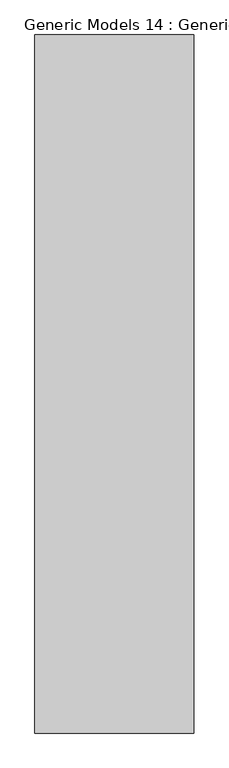
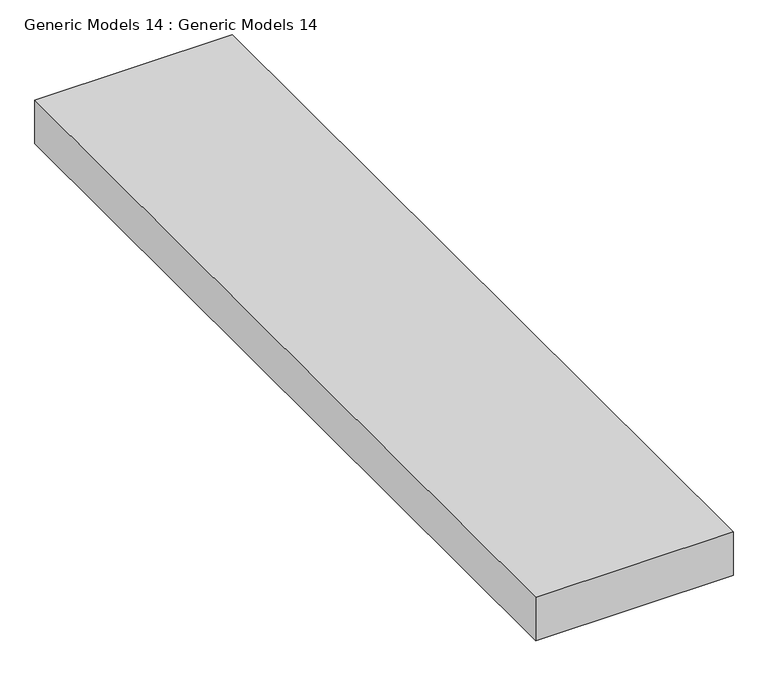
"""IFC4 building model written with IfcOpenShell, lengths in millimetres: proxy geometry, Generic Models 14 : Generic Models 14."""

from ifc_helpers import new_model, si_unit, frame, origin, place, context, project, spatial, polyline, outline, extrude, source, transform, mapped, element, save


def generic_models_14_generic_models_14_04b71fdd(model_context):
    return source(origin(), model_context, "Body", "SweptSolid", [
        extrude(outline(polyline([(-22502.0015274, 2.1945659), (-21845.6161422, 2.1945659), (-21845.6161422, -2882.023242), (-22502.0015274, -2882.023242), (-22502.0015274, 2.1945659)])), frame((0.0, 0.0, 5394.6234092), z_axis=(0.0, 0.0, 1.0), x_axis=(1.0, 0.0, 0.0)), (0.0, 0.0, 1.0), 152.4),
    ])


if __name__ == "__main__":
    model = new_model("IFC4")
    model_context = context("Model", 3, world=origin())
    ifc_project = project(units=[si_unit("LENGTHUNIT", "METRE", prefix="MILLI")], contexts=[model_context])
    site = spatial("IfcSite", under=ifc_project)
    building = spatial("IfcBuilding", under=site)
    placement = place(None, origin())
    generic_models_14_generic_models_14_shape = generic_models_14_generic_models_14_04b71fdd(model_context)
    element("IfcBuildingElementProxy", 1, Name="Generic Models 14 : Generic Models 14", ObjectType="Generic Models 14 : Generic Models 14", at=placement, inside=building, context=model_context, shape_type="MappedRepresentation", body=[
        mapped(generic_models_14_generic_models_14_shape, transform((0.0, 0.0, 0.0), x_axis=(1.0, 0.0, 0.0), y_axis=(0.0, 1.0, 0.0), z_axis=(0.0, 0.0, 1.0))),
    ])
    save(model, "model.ifc")
